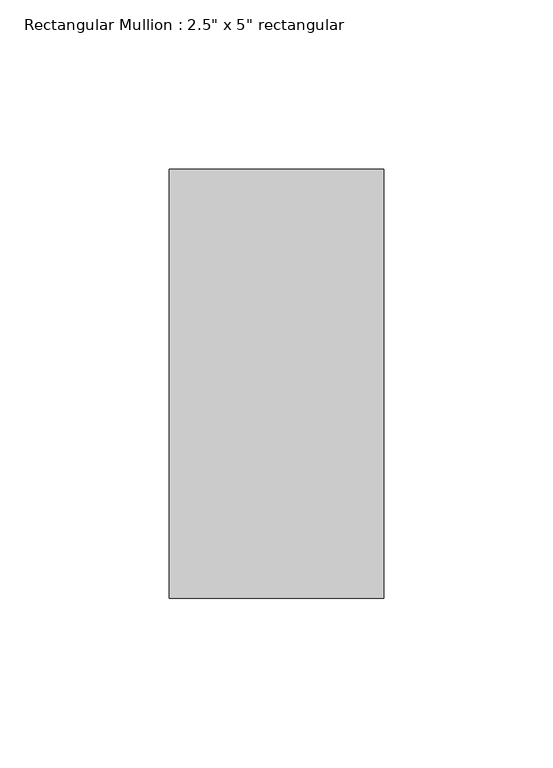
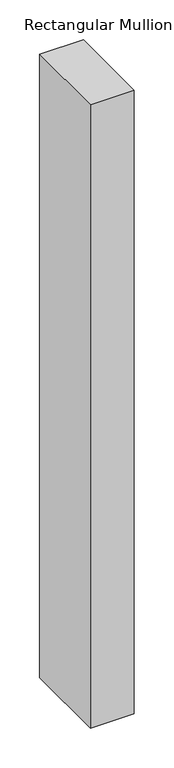
"""IFC4 building model written with IfcOpenShell, lengths in millimetres: member geometry."""

from ifc_helpers import new_model, si_unit, frame, origin, place, context, project, spatial, polyline, outline, extrude, source, transform, mapped, element, save


def member_45f34f4c(model_context):
    return source(origin(), model_context, "Body", "SweptSolid", [
        extrude(outline(polyline([(0.0, 63.5), (0.0, -63.5), (-63.5, -63.5), (-63.5, 63.5), (0.0, 63.5)])), frame((0.0, 0.0, -954.428642), z_axis=(0.0, 0.0, 1.0), x_axis=(1.0, 0.0, 0.0)), (0.0, 0.0, 1.0), 954.428642),
    ])


if __name__ == "__main__":
    model = new_model("IFC4")
    model_context = context("Model", 3, world=origin())
    ifc_project = project(units=[si_unit("LENGTHUNIT", "METRE", prefix="MILLI")], contexts=[model_context])
    site = spatial("IfcSite", under=ifc_project)
    building = spatial("IfcBuilding", under=site)
    placement = place(None, origin())
    member_shape = member_45f34f4c(model_context)
    element("IfcMember", 1, ObjectType="Rectangular Mullion : 2.5\" x 5\" rectangular", at=placement, inside=building, context=model_context, shape_type="MappedRepresentation", body=[
        mapped(member_shape, transform((0.0, 0.0, 0.0), x_axis=(1.0, 0.0, 0.0), y_axis=(0.0, 1.0, 0.0), z_axis=(0.0, 0.0, 1.0))),
    ])
    save(model, "model.ifc")

# Revit data of these elements
# Type "Rectangular Mullion : 2.5\" x 5\" rectangular"
#   built-in parameter 1007304 = 0.416667 (stored number, unit not read)
#   built-in parameter 1007301 = 0.104167 (stored number, unit not read)
#   built-in parameter 1007300 = 0.104167 (stored number, unit not read)
# Element 1 (IfcMember, "Rectangular Mullion : 2.5\" x 5\" rectangular")
#   Materials on its faces: "Aluminum"
# Materials
#   "Aluminum": class "Metal", colour RGB 247 247 247, transparency 0, Description = "Aluminum 6061", Cost = 0
